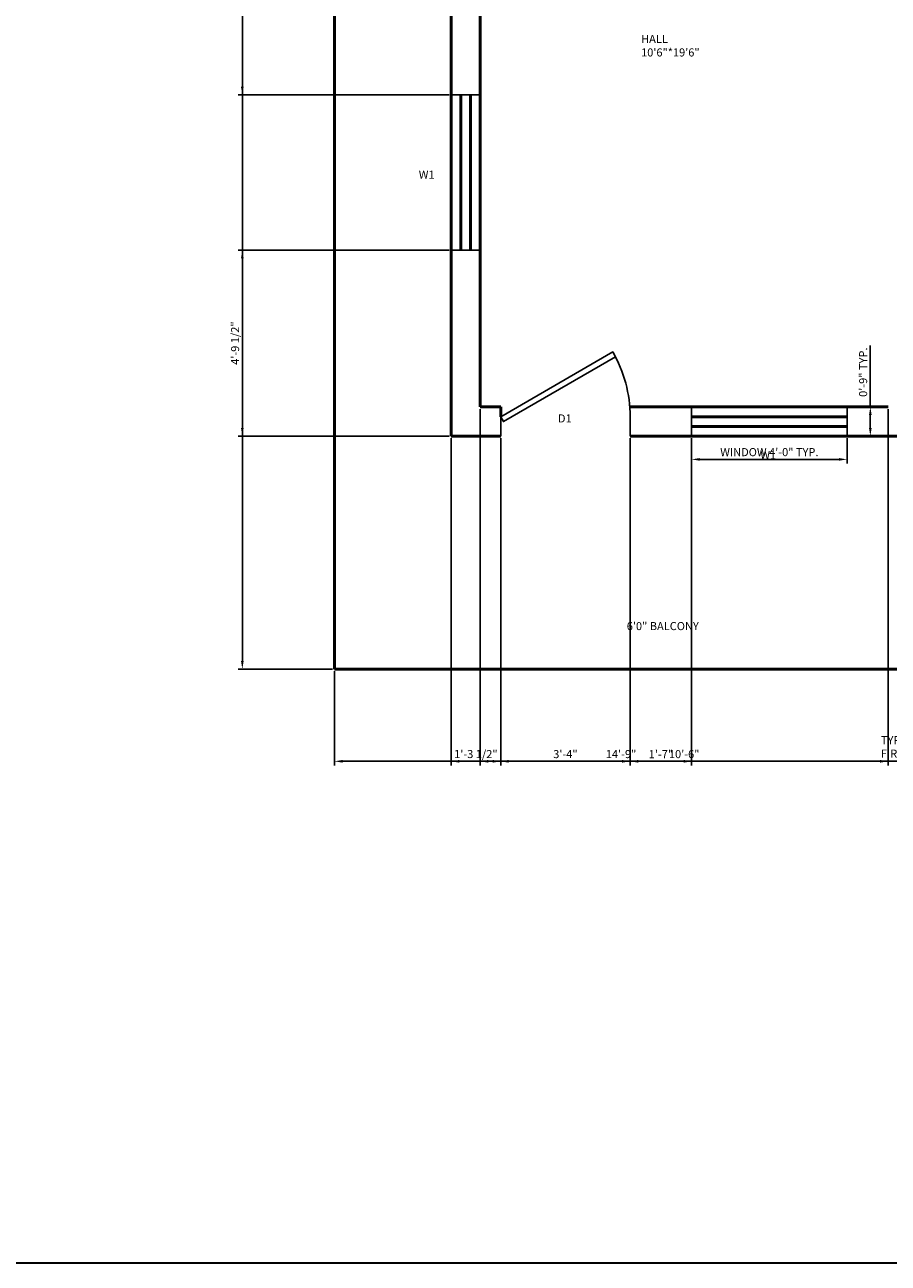
# Model space of a CAD drawing. Units: inches. Extents: x 2020 to 7901, y 1581 to 3943.
# Tile 9 of 17: x 2875 to 3141, y 1581 to 1963. Entities that reach past the tile are written whole.
import ezdxf

# ---------------------------------------------------------------- set-up
doc = ezdxf.new("R2010")
doc.units = ezdxf.units.IN
for name, color, linetype, lineweight in [('A-ANNO-DIMS', 2, 'Continuous', 18), ('A-ANNO-TEXT', 7, 'Continuous', 18), ('A-ANNO-TTLB', 7, 'Continuous', 35), ('A-AREA-IDEN', 3, 'Continuous', 18), ('A-DOOR', 4, 'Continuous', 25), ('A-GLAZ', 4, 'Continuous', 25), ('A-WALL', 7, 'Continuous', 50)]:
    doc.layers.add(name, color=color, linetype=linetype, lineweight=lineweight)
doc.styles.get("Standard").update_dxf_attribs({"font": 'arial.ttf'})
doc.dimstyles.new('ISO-25', dxfattribs={"dimtxt": 2.5, "dimasz": 2.5, "dimexe": 1.25, "dimexo": 0.625, "dimtad": 1, "dimdec": 1, "dimlunit": 3, "dimtxsty": 'Standard', "dimcen": 2.5, "dimadec": 0, "dimazin": 0, "dimtfac": 1, "dimtdec": 1, "dimtmove": 0, "dimatfit": 3, "dimfxl": 1, "dimarcsym": 0})

# ---------------------------------------------------------------- blocks, each defined once
blk = doc.blocks.new('*U9')
for p, q in [((0, 0), (0, -6)), ((40, 0), (40, -6))]:
    blk.add_line(p, q)
blk.add_lwpolyline([(0, 0), (34.64, 20), (35.52, 18.48), (0.87, -1.52)], close=True)
blk.add_arc((0, 0), 40, 0, 30)
blk = doc.blocks.new('WIN-1200')
for p, q in [((0, 9), (48, 9)), ((0, 0), (0, 9)), ((48, 9), (48, 0)), ((48, 0), (0, 0))]:
    blk.add_line(p, q)
blk = doc.blocks.new('*D25')
at = {"layer": 'A-ANNO-DIMS', "color": 0, "lineweight": -2, "transparency": 16777216}
for p, q in [((3080.63, 1835.71), (3080.63, 1827.89)), ((3128.63, 1835.71), (3128.63, 1827.89)), ((3083.13, 1829.14), (3126.13, 1829.14))]:
    blk.add_line(p, q, dxfattribs=at)
at = {"layer": 'A-ANNO-DIMS', "color": 0, "transparency": 16777216}
for points in [[(3083.13, 1829.56), (3083.13, 1828.72), (3080.63, 1829.14)], [(3126.13, 1829.56), (3126.13, 1828.72), (3128.63, 1829.14)]]:
    blk.add_solid(points, dxfattribs=at)
at = {"layer": 'DEFPOINTS', "color": 0, "transparency": 16777216}
for p in [(3080.63, 1836.34), (3128.63, 1836.34), (3128.63, 1829.14)]:
    blk.add_point(p, dxfattribs=at)
at = {"layer": 'A-ANNO-DIMS', "color": 0, "transparency": 16777216, "insert": (3104.63, 1831.06), "char_height": 2.5, "attachment_point": 5}
blk.add_mtext('WINDOW 4\'-0" TYP.', dxfattribs=at)
blk = doc.blocks.new('*D26')
at = {"layer": 'A-ANNO-DIMS', "color": 0, "lineweight": -2, "transparency": 16777216}
for p, q in [((3135.83, 1845.34), (3135.83, 1864.33)), ((3129.26, 1845.34), (3137.08, 1845.34)), ((3135.83, 1838.84), (3135.83, 1842.84)), ((3129.26, 1836.34), (3137.08, 1836.34))]:
    blk.add_line(p, q, dxfattribs=at)
at = {"layer": 'A-ANNO-DIMS', "color": 0, "transparency": 16777216}
for points in [[(3135.42, 1842.84), (3136.25, 1842.84), (3135.83, 1845.34)], [(3135.42, 1838.84), (3136.25, 1838.84), (3135.83, 1836.34)]]:
    blk.add_solid(points, dxfattribs=at)
at = {"layer": 'DEFPOINTS', "color": 0, "transparency": 16777216}
for p in [(3128.63, 1845.34), (3135.83, 1845.34), (3128.63, 1836.34)]:
    blk.add_point(p, dxfattribs=at)
at = {"layer": 'A-ANNO-DIMS', "color": 0, "transparency": 16777216, "insert": (3133.93, 1856.08), "char_height": 2.5, "attachment_point": 5, "rotation": 90}
blk.add_mtext('0\'-9" TYP.', dxfattribs=at)
blk = doc.blocks.new('*D51')
at = {"layer": 'A-ANNO-DIMS', "color": 0, "lineweight": -2, "transparency": 16777216}
for p, q in [((2970.32, 1763.71), (2970.32, 1734.59)), ((3147.32, 1763.71), (3147.32, 1734.59)), ((2972.82, 1735.84), (3144.82, 1735.84))]:
    blk.add_line(p, q, dxfattribs=at)
at = {"layer": 'A-ANNO-DIMS', "color": 0, "transparency": 16777216}
for points in [[(2972.82, 1736.26), (2972.82, 1735.42), (2970.32, 1735.84)], [(3144.82, 1736.26), (3144.82, 1735.42), (3147.32, 1735.84)]]:
    blk.add_solid(points, dxfattribs=at)
at = {"layer": 'DEFPOINTS', "color": 0, "transparency": 16777216}
for p in [(2970.32, 1764.34), (3147.32, 1764.34), (3147.32, 1735.84)]:
    blk.add_point(p, dxfattribs=at)
at = {"layer": 'A-ANNO-DIMS', "color": 0, "transparency": 16777216, "insert": (3058.82, 1737.74), "char_height": 2.5, "attachment_point": 5}
blk.add_mtext('14\'-9"', dxfattribs=at)
blk = doc.blocks.new('*D55')
at = {"layer": 'A-ANNO-DIMS', "color": 0, "lineweight": -2, "transparency": 16777216}
for p, q in [((2969.69, 2240.34), (2940.57, 2240.34)), ((2941.82, 2237.84), (2941.82, 1766.84)), ((2969.69, 1764.34), (2940.57, 1764.34))]:
    blk.add_line(p, q, dxfattribs=at)
at = {"layer": 'A-ANNO-DIMS', "color": 0, "transparency": 16777216}
for points in [[(2941.4, 2237.84), (2942.23, 2237.84), (2941.82, 2240.34)], [(2941.4, 1766.84), (2942.23, 1766.84), (2941.82, 1764.34)]]:
    blk.add_solid(points, dxfattribs=at)
at = {"layer": 'DEFPOINTS', "color": 0, "transparency": 16777216}
for p in [(2970.32, 2240.34), (2941.82, 1764.34), (2970.32, 1764.34)]:
    blk.add_point(p, dxfattribs=at)
at = {"layer": 'A-ANNO-DIMS', "color": 0, "transparency": 16777216, "insert": (2939.91, 2002.34), "char_height": 2.5, "attachment_point": 5, "rotation": 90}
blk.add_mtext('39\'-8"', dxfattribs=at)
blk = doc.blocks.new('*D57')
at = {"layer": 'A-ANNO-DIMS', "color": 0, "lineweight": -2, "transparency": 16777216}
for p, q in [((3021.63, 1835.71), (3021.63, 1734.59)), ((3061.63, 1835.71), (3061.63, 1734.59)), ((3024.13, 1735.84), (3059.13, 1735.84))]:
    blk.add_line(p, q, dxfattribs=at)
at = {"layer": 'A-ANNO-DIMS', "color": 0, "transparency": 16777216}
for points in [[(3024.13, 1736.26), (3024.13, 1735.42), (3021.63, 1735.84)], [(3059.13, 1736.26), (3059.13, 1735.42), (3061.63, 1735.84)]]:
    blk.add_solid(points, dxfattribs=at)
at = {"layer": 'DEFPOINTS', "color": 0, "transparency": 16777216}
for p in [(3021.63, 1836.34), (3061.63, 1836.34), (3061.63, 1735.84)]:
    blk.add_point(p, dxfattribs=at)
at = {"layer": 'A-ANNO-DIMS', "color": 0, "transparency": 16777216, "insert": (3041.63, 1737.74), "char_height": 2.5, "attachment_point": 5}
blk.add_mtext('3\'-4"', dxfattribs=at)
blk = doc.blocks.new('*D128')
at = {"layer": 'A-ANNO-DIMS', "color": 0, "lineweight": -2, "transparency": 16777216}
for p, q in [((3015.32, 1844.71), (3015.32, 1734.59)), ((3141.33, 1844.71), (3141.33, 1734.59)), ((3017.82, 1735.84), (3138.83, 1735.84))]:
    blk.add_line(p, q, dxfattribs=at)
at = {"layer": 'A-ANNO-DIMS', "color": 0, "transparency": 16777216}
for points in [[(3017.82, 1736.26), (3017.82, 1735.42), (3015.32, 1735.84)], [(3138.83, 1736.26), (3138.83, 1735.42), (3141.33, 1735.84)]]:
    blk.add_solid(points, dxfattribs=at)
at = {"layer": 'DEFPOINTS', "color": 0, "transparency": 16777216}
for p in [(3015.32, 1845.34), (3141.33, 1845.34), (3141.33, 1735.84)]:
    blk.add_point(p, dxfattribs=at)
at = {"layer": 'A-ANNO-DIMS', "color": 0, "transparency": 16777216, "insert": (3078.32, 1737.74), "char_height": 2.5, "attachment_point": 5}
blk.add_mtext('10\'-6"', dxfattribs=at)
blk = doc.blocks.new('*D138')
at = {"layer": 'A-ANNO-DIMS', "color": 0, "lineweight": -2, "transparency": 16777216}
for p, q in [((3006.32, 1835.71), (3006.32, 1734.59)), ((3021.63, 1835.71), (3021.63, 1734.59)), ((3008.82, 1735.84), (3019.13, 1735.84))]:
    blk.add_line(p, q, dxfattribs=at)
at = {"layer": 'A-ANNO-DIMS', "color": 0, "transparency": 16777216}
for points in [[(3008.82, 1736.26), (3008.82, 1735.42), (3006.32, 1735.84)], [(3019.13, 1736.26), (3019.13, 1735.42), (3021.63, 1735.84)]]:
    blk.add_solid(points, dxfattribs=at)
at = {"layer": 'DEFPOINTS', "color": 0, "transparency": 16777216}
for p in [(3006.32, 1836.34), (3021.63, 1836.34), (3021.63, 1735.84)]:
    blk.add_point(p, dxfattribs=at)
at = {"layer": 'A-ANNO-DIMS', "color": 0, "transparency": 16777216, "insert": (3013.97, 1737.76), "char_height": 2.5, "attachment_point": 5}
blk.add_mtext('1\'-3 1/2"', dxfattribs=at)
blk = doc.blocks.new('*D139')
at = {"layer": 'A-ANNO-DIMS', "color": 0, "lineweight": -2, "transparency": 16777216}
for p, q in [((3061.63, 1835.71), (3061.63, 1734.59)), ((3080.63, 1835.71), (3080.63, 1734.59)), ((3064.13, 1735.84), (3078.13, 1735.84))]:
    blk.add_line(p, q, dxfattribs=at)
at = {"layer": 'A-ANNO-DIMS', "color": 0, "transparency": 16777216}
for points in [[(3064.13, 1736.26), (3064.13, 1735.42), (3061.63, 1735.84)], [(3078.13, 1736.26), (3078.13, 1735.42), (3080.63, 1735.84)]]:
    blk.add_solid(points, dxfattribs=at)
at = {"layer": 'DEFPOINTS', "color": 0, "transparency": 16777216}
for p in [(3061.63, 1836.34), (3080.63, 1836.34), (3080.63, 1735.84)]:
    blk.add_point(p, dxfattribs=at)
at = {"layer": 'A-ANNO-DIMS', "color": 0, "transparency": 16777216, "insert": (3071.13, 1737.72), "char_height": 2.5, "attachment_point": 5}
blk.add_mtext('1\'-7"', dxfattribs=at)
blk = doc.blocks.new('*D143')
at = {"layer": 'A-ANNO-DIMS', "color": 0, "lineweight": -2, "transparency": 16777216}
for p, q in [((3005.69, 2013.3), (2940.57, 2013.3)), ((2941.82, 2010.8), (2941.82, 1944.29)), ((3005.69, 1941.79), (2940.57, 1941.79))]:
    blk.add_line(p, q, dxfattribs=at)
at = {"layer": 'A-ANNO-DIMS', "color": 0, "transparency": 16777216}
for points in [[(2941.4, 2010.8), (2942.23, 2010.8), (2941.82, 2013.3)], [(2941.4, 1944.29), (2942.23, 1944.29), (2941.82, 1941.79)]]:
    blk.add_solid(points, dxfattribs=at)
at = {"layer": 'DEFPOINTS', "color": 0, "transparency": 16777216}
for p in [(3006.32, 2013.3), (2941.82, 1941.79), (3006.32, 1941.79)]:
    blk.add_point(p, dxfattribs=at)
at = {"layer": 'A-ANNO-DIMS', "color": 0, "transparency": 16777216, "insert": (2939.9, 1977.54), "char_height": 2.5, "attachment_point": 5, "rotation": 90}
blk.add_mtext('5\'-11 1/2"', dxfattribs=at)
blk = doc.blocks.new('*D144')
at = {"layer": 'A-ANNO-DIMS', "color": 0, "lineweight": -2, "transparency": 16777216}
for p, q in [((3005.69, 1893.79), (2940.57, 1893.79)), ((2941.82, 1891.29), (2941.82, 1838.84)), ((3005.69, 1836.34), (2940.57, 1836.34))]:
    blk.add_line(p, q, dxfattribs=at)
at = {"layer": 'A-ANNO-DIMS', "color": 0, "transparency": 16777216}
for points in [[(2941.4, 1891.29), (2942.23, 1891.29), (2941.82, 1893.79)], [(2941.4, 1838.84), (2942.23, 1838.84), (2941.82, 1836.34)]]:
    blk.add_solid(points, dxfattribs=at)
at = {"layer": 'DEFPOINTS', "color": 0, "transparency": 16777216}
for p in [(3006.32, 1893.79), (2941.82, 1836.34), (3006.32, 1836.34)]:
    blk.add_point(p, dxfattribs=at)
at = {"layer": 'A-ANNO-DIMS', "color": 0, "transparency": 16777216, "insert": (2939.9, 1865.07), "char_height": 2.5, "attachment_point": 5, "rotation": 90}
blk.add_mtext('4\'-9 1/2"', dxfattribs=at)

msp = doc.modelspace()

# ---------------------------------------------------------------- linework, layer by layer
at = {"layer": 'A-ANNO-TTLB'}
msp.add_lwpolyline([(2019.8, 3067.25), (4199.03, 3067.25), (4199.03, 1580.73), (2019.8, 1580.73)], close=True, dxfattribs=at)
at = {"layer": 'A-WALL'}
for p, q in [((2970.32, 2214.34), (2970.32, 1836.34)), ((3006.36, 2161.44), (3006.36, 1836.34)), ((3015.32, 2162.04), (3015.32, 1845.34)), ((3009.32, 1893.79), (3009.32, 1941.79)), ((3012.32, 1941.79), (3012.32, 1893.79)), ((3006.32, 1845.34), (3006.36, 1845.34)), ((3015.32, 1845.34), (3021.63, 1845.34)), ((3021.63, 1842.34), (3021.63, 1845.34)), ((3061.51, 1845.34), (3141.33, 1845.34)), ((3080.63, 1842.34), (3128.63, 1842.34)), ((3128.63, 1839.34), (3080.63, 1839.34)), ((2970.32, 1836.34), (2970.32, 1764.34)), ((3006.32, 1836.34), (3021.63, 1836.34)), ((3061.63, 1836.34), (3303.32, 1836.34)), ((2970.32, 1764.34), (3303.32, 1764.34))]:
    msp.add_line(p, q, dxfattribs=at)

# ---------------------------------------------------------------- block references
at = {"layer": 'A-DOOR'}
msp.add_blockref('*U9', (3021.63, 1842.34), dxfattribs=at)
at = {"layer": 'A-GLAZ', "rotation": 90.00000000000003}
msp.add_blockref('WIN-1200', (3015.32, 1893.79), dxfattribs=at)
at = {"layer": 'A-GLAZ'}
msp.add_blockref('WIN-1200', (3080.63, 1836.34), dxfattribs=at)

# ---------------------------------------------------------------- texts
at = {"layer": 'A-ANNO-TEXT', "char_height": 2.5, "attachment_point": 1}
for s, width, insert in [('W1', 8.4295, (2996.32, 1918.39)), ('D1', 9.3529, (3039.32, 1843.05)), ('W1', 20.7227, (3101.85, 1831.75)), ('6\'0" BALCONY', 83.2211, (3060.58, 1778.88)), ('TYPICAL FLOOR PLAN\\PFIRST FLOOR & SECOND FLOOR PLAN', 248.2469, (3139.1, 1743.63))]:
    msp.add_mtext_dynamic_manual_height_columns(s, width=width, gutter_width=12.5, heights=[0], dxfattribs=dict(at, insert=insert))
at = {"layer": 'A-AREA-IDEN', "insert": (3065.01, 1960.32), "char_height": 2.5, "attachment_point": 1}
msp.add_mtext_dynamic_manual_height_columns('HALL\\P10\'6"*19\'6"', width=83.2902, gutter_width=12.5, heights=[0], dxfattribs=at)

# ---------------------------------------------------------------- dimensions: what is measured, and where the dimension line sits
at = {"layer": 'A-ANNO-DIMS'}
for base, p1, p2, picture, middle in [((2941.82, 1764.34), (2970.32, 2240.34), (2970.32, 1764.34), '*D55', (2939.91, 2002.34)), ((2941.82, 1941.79), (3006.32, 2013.3), (3006.32, 1941.79), '*D143', (2939.9, 1977.54)), ((2941.8165, 1836.3394), (3006.3165, 1893.793), (3006.3165, 1836.3394), '*D144', (2939.8989, 1865.0662))]:
    dim = msp.add_linear_dim(base=base, p1=p1, p2=p2, angle=90, dimstyle='ISO-25', override={"dimdec": 1, "dimlfac": 1, "dimrnd": 0, "dimzin": 1, "dimdsep": 46, "dimlunit": 4, "dimfrac": 2}, dxfattribs=at)
    dim.commit()
    dim.dimension.update_dxf_attribs({"geometry": picture, "text_midpoint": middle})
dim = msp.add_linear_dim(base=(3135.83, 1845.34), p1=(3128.63, 1836.34), p2=(3128.63, 1845.34), angle=90, text='<> TYP.', dimstyle='ISO-25', override={"dimdec": 1, "dimrnd": 0, "dimzin": 1, "dimlunit": 4, "dimfrac": 2}, dxfattribs=at)
dim.commit()
dim.dimension.update_dxf_attribs({"geometry": '*D26', "text_midpoint": (3133.93, 1856.08)})
for base, p1, p2, picture, middle in [((3141.33, 1735.84), (3015.32, 1845.34), (3141.33, 1845.34), '*D128', (3078.32, 1737.74)), ((3021.63, 1735.84), (3006.32, 1836.34), (3021.63, 1836.34), '*D138', (3013.97, 1737.76)), ((3061.63, 1735.84), (3021.63, 1836.34), (3061.63, 1836.34), '*D57', (3041.63, 1737.74)), ((3080.63, 1735.84), (3061.63, 1836.34), (3080.63, 1836.34), '*D139', (3071.13, 1737.72)), ((3147.32, 1735.84), (2970.32, 1764.34), (3147.32, 1764.34), '*D51', (3058.82, 1737.74))]:
    dim = msp.add_linear_dim(base=base, p1=p1, p2=p2, dimstyle='ISO-25', override={"dimdec": 1, "dimlfac": 1, "dimrnd": 0, "dimzin": 1, "dimdsep": 46, "dimlunit": 4, "dimfrac": 2}, dxfattribs=at)
    dim.commit()
    dim.dimension.update_dxf_attribs({"geometry": picture, "text_midpoint": middle})
dim = msp.add_linear_dim(base=(3128.63, 1829.14), p1=(3080.63, 1836.34), p2=(3128.63, 1836.34), text='WINDOW <> TYP.', dimstyle='ISO-25', override={"dimdec": 1, "dimrnd": 0, "dimzin": 1, "dimlunit": 4, "dimfrac": 2}, dxfattribs=at)
dim.commit()
dim.dimension.update_dxf_attribs({"geometry": '*D25', "text_midpoint": (3104.63, 1831.06)})

doc.saveas('drawing.dxf')
